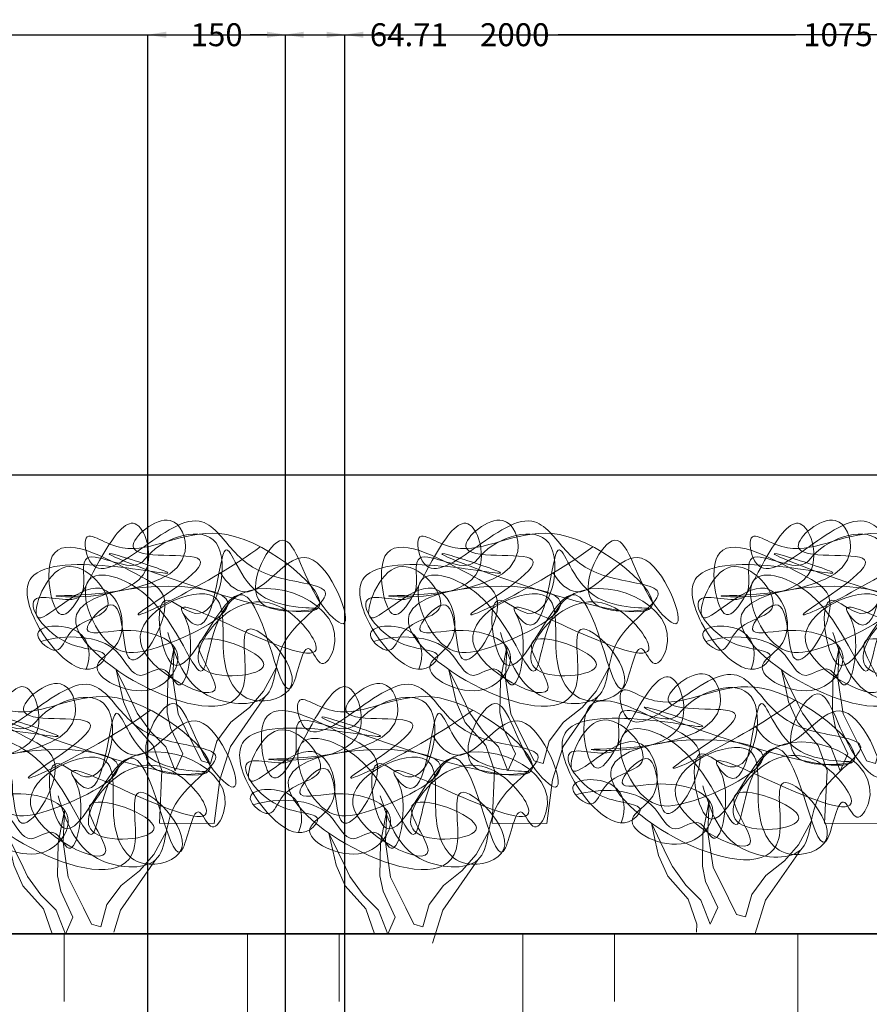
# Model space of a CAD drawing. Units: millimetres. Extents: x -692 to 9639, y -141 to 10345.
# Tile 16 of 19: x 3652 to 4578, y 9272 to 10345. Entities that reach past the tile are written whole.
import ezdxf

# ---------------------------------------------------------------- set-up
doc = ezdxf.new("R2010")
doc.units = ezdxf.units.MM
doc.header["$MEASUREMENT"] = 0
for name, color, linetype, lineweight in [('A-ANNO-DIMS', 2, 'Continuous', 18), ('A-ELEV', 7, 'Continuous', 35), ('A-ELEV-PATT', 8, 'Continuous', 13), ('L-PLNT', 3, 'Continuous', 18)]:
    doc.layers.add(name, color=color, linetype=linetype, lineweight=lineweight)
doc.styles.get("Standard").update_dxf_attribs({"font": 'arial.ttf'})
doc.dimstyles.get("Standard").update_dxf_attribs({"dimtxt": 25, "dimasz": 20, "dimexe": 0.18, "dimexo": 10, "dimgap": 10, "dimtad": 0, "dimtih": 1, "dimtoh": 1, "dimdec": 0, "dimzin": 0, "dimdsep": 46, "dimtxsty": 'Standard', "dimcen": 10, "dimadec": 0, "dimazin": 0, "dimtfac": 1, "dimtdec": 0, "dimtofl": 0, "dimtmove": 0, "dimatfit": 3, "dimfxl": 1, "dimtolj": 1, "dimtzin": 0, "dimarcsym": 0})

# ---------------------------------------------------------------- blocks, each defined once
blk = doc.blocks.new('SHRUB-A')
for p, q in [((56.2, 156.7), (63.1, 192.4)), ((63.1, 192.4), (61.6, 157.6)), ((4.3, 148.6), (0, 167.6)), ((0, 167.6), (10, 146.8)), ((160.6, 144.2), (174.3, 169.5)), ((55.6, 120.9), (56.2, 156.7)), ((61.6, 157.6), (67.3, 119.6)), ((7.9, 132.5), (4.3, 148.6)), ((10, 146.8), (18, 130.3)), ((145.1, 126.5), (160.6, 144.2)), ((17.8, 109.9), (7.9, 132.5)), ((18, 130.3), (22.9, 120.3)), ((162.4, 138.4), (124.4, 83.7)), ((22.9, 120.3), (37.4, 100.1)), ((59.1, 104.1), (55.6, 120.9)), ((67.3, 119.6), (83.9, 86)), ((124.8, 110.5), (145.1, 126.5)), ((40.2, 84.8), (17.8, 109.9)), ((109.4, 89.7), (124.8, 110.5)), ((37.4, 100.1), (54, 83.6)), ((72.4, 75.8), (59.1, 104.1)), ((83.9, 86), (92.7, 68.2)), ((102.6, 65.4), (109.4, 89.7)), ((49.7, 57.7), (40.2, 84.8)), ((54, 83.6), (64.1, 57.4)), ((64.1, 57.4), (72.4, 75.8)), ((124.4, 83.7), (113, 47.4)), ((92.7, 68.2), (102.6, 65.4)), ((47, 0.4), (49.7, 57.7)), ((113, 47.4), (106.7, 0)), ((106.7, 0), (47, 0.4))]:
    blk.add_line(p, q)
blk = doc.blocks.new('SHRUB-B')
for p, q in [((56.2, 99.2), (63.1, 135)), ((63.1, 135), (61.6, 100.2)), ((4.3, 91.2), (0, 110.2)), ((0, 110.2), (10, 89.4)), ((160.6, 86.8), (174.3, 112.1)), ((55.6, 63.5), (56.2, 99.2)), ((61.6, 100.2), (67.3, 62.2)), ((7.9, 75.1), (4.3, 91.2)), ((10, 89.4), (18, 72.9)), ((145.1, 69.1), (160.6, 86.8)), ((17.8, 52.5), (7.9, 75.1)), ((18, 72.9), (22.9, 62.9)), ((124.8, 53.1), (145.1, 69.1)), ((22.9, 62.9), (37.4, 42.7)), ((59.1, 46.7), (55.6, 63.5)), ((67.3, 62.2), (83.9, 28.6)), ((40.2, 27.4), (17.8, 52.5)), ((72.4, 18.4), (59.1, 46.7)), ((109.4, 32.3), (124.8, 53.1)), ((37.4, 42.7), (54, 26.2)), ((102.6, 8), (109.4, 32.3)), ((49.7, 0.3), (40.2, 27.4)), ((54, 26.2), (64.1, 0)), ((83.9, 28.6), (92.7, 10.8)), ((64.1, 0), (72.4, 18.4)), ((92.7, 10.8), (102.6, 8))]:
    blk.add_line(p, q)
blk = doc.blocks.new('*D7')
at = {"layer": 'A-ANNO-DIMS', "color": 0, "lineweight": -2, "transparency": 16777216}
for p, q in [((8481.5, 9848.8), (-649.1, 9848.8)), ((-648.9, 9828.8), (-648.9, 5124.9)), ((-648.9, 375.6), (-648.9, 5079.4)), ((2463.7, 355.6), (-649.1, 355.6))]:
    blk.add_line(p, q, dxfattribs=at)
at = {"layer": 'A-ANNO-DIMS', "color": 0, "lineweight": -3, "transparency": 16777216}
for points in [[(-652.2, 9828.8), (-645.6, 9828.8), (-648.9, 9848.8)], [(-652.2, 375.6), (-645.6, 375.6), (-648.9, 355.6)]]:
    blk.add_solid(points, dxfattribs=at)
at = {"layer": 'Defpoints', "color": 0, "lineweight": -3, "transparency": 16777216}
for p in [(-648.9, 9848.8), (8491.5, 9848.8), (2473.7, 355.6)]:
    blk.add_point(p, dxfattribs=at)
at = {"layer": 'A-ANNO-DIMS', "color": 0, "transparency": 16777216, "insert": (-648.9, 5102.2), "char_height": 25, "attachment_point": 5}
blk.add_mtext('\\A1;9493', dxfattribs=at)
blk = doc.blocks.new('*D14')
at = {"layer": 'A-ANNO-DIMS', "color": 0, "lineweight": -2, "transparency": 16777216}
for p, q in [((3191.5, 9358.8), (3191.5, 10329)), ((3211.5, 10328.8), (4144, 10328.8)), ((5171.5, 10328.8), (4239, 10328.8)), ((5191.5, 9358.8), (5191.5, 10329))]:
    blk.add_line(p, q, dxfattribs=at)
at = {"layer": 'A-ANNO-DIMS', "color": 0, "lineweight": -3, "transparency": 16777216}
for points in [[(3211.5, 10332.1), (3211.5, 10325.4), (3191.5, 10328.8)], [(5171.5, 10332.1), (5171.5, 10325.4), (5191.5, 10328.8)]]:
    blk.add_solid(points, dxfattribs=at)
at = {"layer": 'Defpoints', "color": 0, "lineweight": -3, "transparency": 16777216}
for p in [(5191.5, 10328.8), (3191.5, 9348.8), (5191.5, 9348.8)]:
    blk.add_point(p, dxfattribs=at)
at = {"layer": 'A-ANNO-DIMS', "color": 0, "transparency": 16777216, "insert": (4191.5, 10328.8), "char_height": 25, "attachment_point": 5}
blk.add_mtext('\\A1;2000', dxfattribs=at)
blk = doc.blocks.new('*D52')
at = {"layer": 'A-ANNO-DIMS', "color": 0, "lineweight": -2, "transparency": 16777216}
for p, q in [((3791.5, 6858.8), (3791.5, 10329)), ((3811.5, 10328.8), (3830.1, 10328.8)), ((3921.5, 10328.8), (3902.9, 10328.8)), ((3941.5, 6708.8), (3941.5, 10329))]:
    blk.add_line(p, q, dxfattribs=at)
at = {"layer": 'A-ANNO-DIMS', "color": 0, "lineweight": -3, "transparency": 16777216}
for points in [[(3811.5, 10332.1), (3811.5, 10325.4), (3791.5, 10328.8)], [(3921.5, 10332.1), (3921.5, 10325.4), (3941.5, 10328.8)]]:
    blk.add_solid(points, dxfattribs=at)
at = {"layer": 'Defpoints', "color": 0, "lineweight": -3, "transparency": 16777216}
for p in [(3941.5, 10328.8), (3791.5, 6848.8), (3941.5, 6698.8)]:
    blk.add_point(p, dxfattribs=at)
at = {"layer": 'A-ANNO-DIMS', "color": 0, "transparency": 16777216, "insert": (3866.5, 10328.8), "char_height": 25, "attachment_point": 5}
blk.add_mtext('\\A1;150', dxfattribs=at)
blk = doc.blocks.new('*D53')
at = {"layer": 'A-ANNO-DIMS', "color": 0, "lineweight": -2, "transparency": 16777216}
for p, q in [((3941.5, 6708.8), (3941.5, 10329)), ((3961.5, 10328.8), (3986.3, 10328.8)), ((4006.3, 6433.8), (4006.3, 10329)), ((4006.3, 10328.8), (4026.3, 10328.8))]:
    blk.add_line(p, q, dxfattribs=at)
at = {"layer": 'A-ANNO-DIMS', "color": 0, "lineweight": -3, "transparency": 16777216}
for points in [[(3961.5, 10332.1), (3961.5, 10325.4), (3941.5, 10328.8)], [(3986.3, 10332.1), (3986.3, 10325.4), (4006.3, 10328.8)]]:
    blk.add_solid(points, dxfattribs=at)
at = {"layer": 'Defpoints', "color": 0, "lineweight": -3, "transparency": 16777216}
for p in [(4006.3, 10328.8), (3941.5, 6698.8), (4006.3, 6423.8)]:
    blk.add_point(p, dxfattribs=at)
at = {"layer": 'A-ANNO-DIMS', "color": 0, "transparency": 16777216, "insert": (4076.1, 10328.8), "char_height": 25, "attachment_point": 5}
blk.add_mtext('\\A1;64.71', dxfattribs=at)
blk = doc.blocks.new('*D54')
at = {"layer": 'A-ANNO-DIMS', "color": 0, "lineweight": -2, "transparency": 16777216}
for p, q in [((4006.3, 6433.8), (4006.3, 10329)), ((4026.3, 10328.8), (4497.5, 10328.8)), ((5061.3, 10328.8), (4590, 10328.8)), ((5081.3, 6433.8), (5081.3, 10329))]:
    blk.add_line(p, q, dxfattribs=at)
at = {"layer": 'A-ANNO-DIMS', "color": 0, "lineweight": -3, "transparency": 16777216}
for points in [[(4026.3, 10332.1), (4026.3, 10325.4), (4006.3, 10328.8)], [(5061.3, 10332.1), (5061.3, 10325.4), (5081.3, 10328.8)]]:
    blk.add_solid(points, dxfattribs=at)
at = {"layer": 'Defpoints', "color": 0, "lineweight": -3, "transparency": 16777216}
for p in [(5081.3, 10328.8), (4006.3, 6423.8), (5081.3, 6423.8)]:
    blk.add_point(p, dxfattribs=at)
at = {"layer": 'A-ANNO-DIMS', "color": 0, "transparency": 16777216, "insert": (4543.8, 10328.8), "char_height": 25, "attachment_point": 5}
blk.add_mtext('\\A1;1075', dxfattribs=at)

msp = doc.modelspace()

# ---------------------------------------------------------------- hatches: boundary and pattern name
at = {"layer": 'A-ELEV-PATT'}
h = msp.add_hatch(dxfattribs=at)
h.set_pattern_fill('GOST_WOOD', color=256, scale=50)
h.set_pattern_definition([(90, (0, 0), (300, -2e-14), [500, -100]), (90, (100, -100), (300, -2e-14), [300, -75, 150, -75]), (90, (200, -250), (300, -2e-14), [500, -100])])
edge = h.paths.add_edge_path()
edge.add_line((5191.547, 8748.772), (3791.547, 8748.772))
edge.add_line((3791.547, 8748.772), (3791.547, 8848.772))
edge.add_line((3791.547, 8848.772), (5191.547, 8848.772))
edge.add_line((5191.547, 8848.772), (5191.547, 9348.772))
edge.add_line((5191.547, 9348.772), (4755.992, 9348.772))
edge.add_line((4755.992, 9348.772), (4755.854, 9348.465))
edge.add_line((4755.854, 9348.465), (4755.734, 9348.772))
edge.add_line((4755.734, 9348.772), (4053.129, 9348.772))
edge.add_line((4053.129, 9348.772), (4052.99, 9348.465))
edge.add_line((4052.99, 9348.465), (4052.871, 9348.772))
edge.add_line((4052.871, 9348.772), (3701.731, 9348.772))
edge.add_line((3701.731, 9348.772), (3701.593, 9348.465))
edge.add_line((3701.593, 9348.465), (3701.474, 9348.772))
edge.add_line((3701.474, 9348.772), (3368.199, 9348.772))
edge.add_line((3368.199, 9348.772), (3368.061, 9348.465))
edge.add_line((3368.061, 9348.465), (3367.942, 9348.772))
edge.add_line((3367.942, 9348.772), (3191.547, 9348.772))
edge.add_line((3191.547, 9348.772), (3191.547, 3210.058))
edge.add_spline(control_points=[(3191.547, 3210.058), (3198.467, 3207.5), (3283.859, 3166.656), (3324.053, 2995.08), (3234.02, 2920.058), (3220.783, 2911.684)], knot_values=[13649.89756952, 13649.89756952, 13649.89756952, 13649.89756952, 13672.14990348, 13935.42377748, 13974.4426778, 13974.4426778, 13974.4426778, 13974.4426778], degree=3, periodic=0)
edge.add_spline(control_points=[(3220.783, 2911.684), (3225.148, 2890.107), (3226.864, 2868.931), (3226.144, 2848.27)], knot_values=[8828.69997321, 8828.69997321, 8828.69997321, 8828.69997321, 8890.6429847, 8890.6429847, 8890.6429847, 8890.6429847], degree=3, periodic=0)
edge.add_line((3226.144, 2848.27), (5191.547, 2848.27))
edge.add_line((5191.547, 2848.27), (5191.547, 3048.27))
edge.add_line((5191.547, 3048.27), (5041.547, 3048.27))
edge.add_line((5041.547, 3048.27), (5041.547, 3148.27))
edge.add_line((5041.547, 3148.27), (5091.547, 3148.27))
edge.add_line((5091.547, 3148.27), (5091.547, 3598.27))
edge.add_line((5091.547, 3598.27), (5191.547, 3598.27))
edge.add_line((5191.547, 3598.27), (5191.547, 4848.772))
edge.add_line((5191.547, 4848.772), (3791.547, 4848.772))
edge.add_line((3791.547, 4848.772), (3791.547, 6848.772))
edge.add_line((3791.547, 6848.772), (5091.547, 6848.772))
edge.add_line((5091.547, 6848.772), (5091.547, 7298.772))
edge.add_line((5091.547, 7298.772), (5191.547, 7298.772))
edge.add_line((5191.547, 7298.772), (5191.547, 8748.772))
h.paths.add_polyline_path([(5016.547, 8198.772), (5016.547, 7123.772), (3941.547, 7123.772), (3941.547, 8198.772)], flags=16)
h.paths.add_polyline_path([(4941.547, 8123.772), (4941.547, 7198.772), (4016.547, 7198.772), (4016.547, 8123.772)], flags=0)
h.paths.add_polyline_path([(4616.547, 8073.772), (4616.547, 7248.772), (4341.547, 7248.772), (4341.547, 8073.772)], flags=0)
h.paths.add_polyline_path([(4641.547, 8073.772), (4891.547, 8073.772), (4891.547, 7248.772), (4641.547, 7248.772)], flags=0)
h.paths.add_polyline_path([(4666.547, 8048.772), (4866.547, 8048.772), (4866.547, 7273.772), (4666.547, 7273.772)], flags=0)
h.paths.add_polyline_path([(4316.547, 8073.772), (4316.547, 7248.772), (4066.547, 7248.772), (4066.547, 8073.772)], flags=0)
h.paths.add_polyline_path([(4291.547, 8048.772), (4291.547, 7273.772), (4091.547, 7273.772), (4091.547, 8048.772)], flags=0)
h.paths.add_polyline_path([(5016.547, 4497.772), (5016.547, 3422.772), (3941.547, 3422.772), (3941.547, 4497.772)], flags=16)
h.paths.add_polyline_path([(4941.547, 4422.772), (4941.547, 3497.772), (4016.547, 3497.772), (4016.547, 4422.772)], flags=0)
h.paths.add_polyline_path([(4616.547, 4372.772), (4616.547, 3547.772), (4341.547, 3547.772), (4341.547, 4372.772)], flags=0)
h.paths.add_polyline_path([(4641.547, 4372.772), (4891.547, 4372.772), (4891.547, 3547.772), (4641.547, 3547.772)], flags=0)
h.paths.add_polyline_path([(4316.547, 4372.772), (4316.547, 3547.772), (4066.547, 3547.772), (4066.547, 4372.772)], flags=0)
h.paths.add_polyline_path([(4666.547, 4347.772), (4866.547, 4347.772), (4866.547, 3572.772), (4666.547, 3572.772)], flags=0)
h.paths.add_polyline_path([(4291.547, 4347.772), (4291.547, 3572.772), (4091.547, 3572.772), (4091.547, 4347.772)], flags=0)

# ---------------------------------------------------------------- linework, layer by layer
at = {"layer": 'A-ELEV'}
msp.add_line((3191.547, 9348.772), (5191.547, 9348.772), dxfattribs=at)
at = {"layer": 'L-PLNT'}
for p, q in [((4396.605, 9458.408), (4403.593, 9494.115)), ((4403.593, 9494.115), (4402.028, 9459.362)), ((4344.728, 9450.331), (4340.453, 9469.321)), ((4340.453, 9469.321), (4350.494, 9448.579)), ((4501.01, 9445.975), (4514.74, 9471.226)), ((4396.049, 9422.669), (4396.605, 9458.408)), ((4402.028, 9459.362), (4407.8, 9421.335)), ((4348.34, 9434.283), (4344.728, 9450.331)), ((4350.494, 9448.579), (4358.483, 9432.077)), ((4485.516, 9428.273), (4501.01, 9445.975)), ((4358.252, 9411.658), (4348.34, 9434.283)), ((4502.899, 9440.134), (4464.833, 9385.403)), ((3799.897, 9429.44), (3761.831, 9374.709)), ((4151.294, 9429.44), (4113.229, 9374.709)), ((4358.483, 9432.077), (4363.315, 9422.096)), ((4465.219, 9412.262), (4485.516, 9428.273)), ((4363.315, 9422.096), (4377.888, 9401.855)), ((4399.52, 9405.858), (4396.049, 9422.669)), ((4407.8, 9421.335), (4424.358, 9387.712)), ((4449.855, 9391.498), (4465.219, 9412.262)), ((4380.638, 9386.579), (4358.252, 9411.658)), ((4377.888, 9401.855), (4394.446, 9385.31)), ((4412.874, 9377.572), (4399.52, 9405.858)), ((4443.052, 9367.164), (4449.855, 9391.498)), ((4390.135, 9359.466), (4380.638, 9386.579)), ((4394.446, 9385.31), (4404.595, 9359.159)), ((4424.358, 9387.712), (4433.107, 9369.945)), ((4464.833, 9385.403), (4453.484, 9349.201)), ((3761.831, 9374.709), (3754.255, 9350.541)), ((4113.229, 9374.709), (4101.88, 9338.507)), ((4404.595, 9359.159), (4412.874, 9377.572)), ((4433.107, 9369.945), (4443.052, 9367.164)), ((4389.721, 9350.541), (4390.135, 9359.466))]:
    msp.add_line(p, q, dxfattribs=at)
for points, knots in [([(3870.787, 9742.239), (3877.292, 9730.903), (3910.528, 9700.951), (3966.958, 9812.559), (4026.138, 9660.867), (3961.502, 9722.363), (3945.777, 9821.568), (3878.818, 9687.955), (4016.284, 9708.276), (3899.439, 9697.909), (3870.103, 9822.951), (3864.501, 9656.273), (3811.999, 9718.176), (3905.68, 9672.588), (4002.746, 9634.5), (3933.585, 9723.816), (3867.431, 9704.087), (3825.22, 9620.458), (3976.108, 9634.855), (3810.499, 9696.668), (3906.873, 9576.858), (3713.031, 9670.533), (3887.727, 9749.582), (3865.518, 9651.408), (3894.256, 9592.145), (3980.508, 9617.027), (3878.674, 9721.539), (3933.88, 9522.359), (3548.286, 9733.486), (3963.38, 9736.751), (3813.397, 9659.817), (3742.545, 9649.423), (3699.733, 9757.262), (3814.514, 9723.536), (3856.602, 9579.097), (3861.587, 9768.661), (4023.281, 9702.629), (3980.554, 9633.263), (3962.517, 9680.84), (3941.722, 9544.945), (3904.968, 9826.86), (3817.837, 9563.572), (3792.835, 9739.876), (3862.604, 9668.929), (3894.271, 9809.339), (3803.73, 9778.979), (3774.605, 9737.949), (3707.662, 9784.348), (3733.853, 9697.774), (3641.411, 9733.91), (3691.228, 9654.8), (3752.747, 9658.957), (3722.581, 9620.328), (3667.277, 9675.174), (3642.995, 9782.065), (3887.369, 9719.852), (3639.078, 9801.027), (4099.827, 9622.054), (3874.162, 9821.297), (3794.319, 9760.575), (3748.016, 9773.261), (3719.932, 9789.116), (3732.294, 9699.252), (3833.622, 9839.527), (3885.762, 9759.776), (3924.577, 9734.293), (4016.253, 9726.404), (3923.236, 9674.075), (3937.396, 9593.308), (3837.579, 9601.408), (3821.952, 9650.09), (3813.209, 9677.329)], [2413.81083439, 2413.81083439, 2413.81083439, 2413.81083439, 2446.13175162, 2525.76080664, 2606.35842411, 2641.00152553, 2720.74212251, 2790.99014926, 2851.81652626, 2913.32865241, 2976.26621652, 3063.90114016, 3082.75198237, 3142.42040078, 3234.21047015, 3290.89514405, 3366.44484787, 3415.98940505, 3483.69911772, 3557.93307926, 3609.73318023, 3705.73947781, 3799.4035149, 3865.9559372, 3923.0506034, 3967.47996902, 4044.49288828, 4106.44083814, 4304.51898163, 4470.20683119, 4567.66187689, 4605.3795614, 4686.71522755, 4750.59418277, 4853.67923318, 4940.38216709, 5061.92671957, 5081.75583403, 5102.38342504, 5145.20608443, 5257.20859169, 5364.77120979, 5434.601162, 5468.93345211, 5548.91442162, 5624.29444335, 5636.24531967, 5696.20028889, 5735.53268567, 5783.76480276, 5846.42206129, 5886.03768999, 5892.5373904, 5975.51315878, 6025.10951571, 6171.93373357, 6229.50952465, 6457.88730992, 6585.61219414, 6694.59236697, 6720.94216912, 6740.48817363, 6762.80712224, 6890.45590486, 6938.76737224, 6996.52597549, 7050.2147859, 7119.04318667, 7183.57042671, 7247.02609863, 7327.63038966, 7327.63038966, 7327.63038966, 7327.63038966]), ([(3724.096, 9637.137), (3730.159, 9651.341), (3726.664, 9689.445), (3652.093, 9684.583), (3695.541, 9647.305), (3706.222, 9691.38), (3775.283, 9694.456), (3695.331, 9786.768), (3646.836, 9649.897), (3745.311, 9765.156), (3777.086, 9667.558), (3713.033, 9636.75), (3795.836, 9595.485), (3843.182, 9663.04), (3778.736, 9686.864), (3708.195, 9669.411), (3769.699, 9738.522), (3756.754, 9597.689), (3831.066, 9714.368), (3765.302, 9747.322), (3669.526, 9801.44), (3693.692, 9656.882), (3733.265, 9753.527), (3780.402, 9818.105), (3813.993, 9708.231), (3585.245, 9723.215), (3859.393, 9710.208), (3819.392, 9819.441), (3735.993, 9748.74), (3911.027, 9777.439), (3699.503, 9652.419), (3863.756, 9733.103), (3913.888, 9770.678)], [369.05069933, 369.05069933, 369.05069933, 369.05069933, 408.0755152, 451.81999766, 477.70991819, 501.76804774, 551.72688153, 614.71506468, 677.59190345, 752.65992621, 814.92518896, 848.06947292, 911.78367098, 957.89252981, 1028.01014559, 1063.15062915, 1099.93333455, 1162.00574744, 1235.23981988, 1278.45742209, 1371.86548038, 1434.47491944, 1513.90135623, 1562.79289697, 1613.81915843, 1716.27616866, 1864.9556669, 1902.31221643, 1951.61463942, 2025.20033993, 2111.30740148, 2244.75178922, 2244.75178922, 2244.75178922, 2244.75178922]), ([(4233.453, 9742.239), (4239.959, 9730.903), (4273.195, 9700.951), (4329.624, 9812.559), (4388.805, 9660.867), (4324.169, 9722.363), (4308.443, 9821.568), (4241.484, 9687.955), (4378.95, 9708.276), (4262.105, 9697.909), (4232.77, 9822.951), (4227.167, 9656.273), (4174.665, 9718.176), (4268.346, 9672.588), (4365.412, 9634.5), (4296.251, 9723.816), (4230.098, 9704.087), (4187.887, 9620.458), (4338.774, 9634.855), (4173.165, 9696.668), (4269.539, 9576.858), (4075.697, 9670.533), (4250.394, 9749.582), (4228.185, 9651.408), (4256.922, 9592.145), (4343.175, 9617.027), (4241.341, 9721.539), (4296.546, 9522.359), (3910.953, 9733.486), (4326.046, 9736.751), (4176.063, 9659.817), (4105.212, 9649.423), (4062.399, 9757.262), (4177.18, 9723.536), (4219.268, 9579.097), (4224.254, 9768.661), (4385.947, 9702.629), (4343.22, 9633.263), (4325.183, 9680.84), (4304.388, 9544.945), (4267.634, 9826.86), (4180.503, 9563.572), (4155.501, 9739.876), (4225.27, 9668.929), (4256.937, 9809.339), (4166.397, 9778.979), (4137.271, 9737.949), (4070.329, 9784.348), (4096.519, 9697.774), (4004.078, 9733.91), (4053.894, 9654.8), (4115.414, 9658.957), (4085.247, 9620.328), (4029.943, 9675.174), (4005.662, 9782.065), (4250.036, 9719.852), (4001.744, 9801.027), (4462.493, 9622.054), (4236.829, 9821.297), (4156.985, 9760.575), (4110.682, 9773.261), (4082.599, 9789.116), (4094.96, 9699.252), (4196.289, 9839.527), (4248.429, 9759.776), (4287.243, 9734.293), (4378.919, 9726.404), (4285.902, 9674.075), (4300.063, 9593.308), (4200.245, 9601.408), (4184.619, 9650.09), (4175.875, 9677.329)], [2413.81083439, 2413.81083439, 2413.81083439, 2413.81083439, 2446.13175162, 2525.76080664, 2606.35842411, 2641.00152553, 2720.74212251, 2790.99014926, 2851.81652626, 2913.32865241, 2976.26621652, 3063.90114016, 3082.75198237, 3142.42040078, 3234.21047015, 3290.89514405, 3366.44484787, 3415.98940505, 3483.69911772, 3557.93307926, 3609.73318023, 3705.73947781, 3799.4035149, 3865.9559372, 3923.0506034, 3967.47996902, 4044.49288828, 4106.44083814, 4304.51898163, 4470.20683119, 4567.66187689, 4605.3795614, 4686.71522755, 4750.59418277, 4853.67923318, 4940.38216709, 5061.92671957, 5081.75583403, 5102.38342504, 5145.20608443, 5257.20859169, 5364.77120979, 5434.601162, 5468.93345211, 5548.91442162, 5624.29444335, 5636.24531967, 5696.20028889, 5735.53268567, 5783.76480276, 5846.42206129, 5886.03768999, 5892.5373904, 5975.51315878, 6025.10951571, 6171.93373357, 6229.50952465, 6457.88730992, 6585.61219414, 6694.59236697, 6720.94216912, 6740.48817363, 6762.80712224, 6890.45590486, 6938.76737224, 6996.52597549, 7050.2147859, 7119.04318667, 7183.57042671, 7247.02609863, 7327.63038966, 7327.63038966, 7327.63038966, 7327.63038966]), ([(4086.762, 9637.137), (4092.825, 9651.341), (4089.331, 9689.445), (4014.759, 9684.583), (4058.207, 9647.305), (4068.889, 9691.38), (4137.95, 9694.456), (4057.998, 9786.768), (4009.502, 9649.897), (4107.978, 9765.156), (4139.753, 9667.558), (4075.699, 9636.75), (4158.502, 9595.485), (4205.849, 9663.04), (4141.402, 9686.864), (4070.861, 9669.411), (4132.366, 9738.522), (4119.421, 9597.689), (4193.732, 9714.368), (4127.969, 9747.322), (4032.193, 9801.44), (4056.358, 9656.882), (4095.932, 9753.527), (4143.068, 9818.105), (4176.659, 9708.231), (3947.911, 9723.215), (4222.059, 9710.208), (4182.058, 9819.441), (4098.659, 9748.74), (4273.694, 9777.439), (4062.17, 9652.419), (4226.423, 9733.103), (4276.554, 9770.678)], [369.05069933, 369.05069933, 369.05069933, 369.05069933, 408.0755152, 451.81999766, 477.70991819, 501.76804774, 551.72688153, 614.71506468, 677.59190345, 752.65992621, 814.92518896, 848.06947292, 911.78367098, 957.89252981, 1028.01014559, 1063.15062915, 1099.93333455, 1162.00574744, 1235.23981988, 1278.45742209, 1371.86548038, 1434.47491944, 1513.90135623, 1562.79289697, 1613.81915843, 1716.27616866, 1864.9556669, 1902.31221643, 1951.61463942, 2025.20033993, 2111.30740148, 2244.75178922, 2244.75178922, 2244.75178922, 2244.75178922]), ([(4595.897, 9742.239), (4602.402, 9730.903), (4635.638, 9700.951), (4692.068, 9812.559), (4751.248, 9660.867), (4686.612, 9722.363), (4670.887, 9821.568), (4603.928, 9687.955), (4741.394, 9708.276), (4624.549, 9697.909), (4595.213, 9822.951), (4589.611, 9656.273), (4537.109, 9718.176), (4630.79, 9672.588), (4727.856, 9634.5), (4658.695, 9723.816), (4592.541, 9704.087), (4550.33, 9620.458), (4701.218, 9634.855), (4535.609, 9696.668), (4631.983, 9576.858), (4438.141, 9670.533), (4612.837, 9749.582), (4590.628, 9651.408), (4619.366, 9592.145), (4705.618, 9617.027), (4603.784, 9721.539), (4658.99, 9522.359), (4273.396, 9733.486), (4688.49, 9736.751), (4538.507, 9659.817), (4467.655, 9649.423), (4424.843, 9757.262), (4539.624, 9723.536), (4581.712, 9579.097), (4586.697, 9768.661), (4748.391, 9702.629), (4705.664, 9633.263), (4687.627, 9680.84), (4666.832, 9544.945), (4630.078, 9826.86), (4542.947, 9563.572), (4517.945, 9739.876), (4587.714, 9668.929), (4619.381, 9809.339), (4528.84, 9778.979), (4499.715, 9737.949), (4432.772, 9784.348), (4458.963, 9697.774), (4366.521, 9733.91), (4416.338, 9654.8), (4477.857, 9658.957), (4447.691, 9620.328), (4392.387, 9675.174), (4368.105, 9782.065), (4612.479, 9719.852), (4364.188, 9801.027), (4824.937, 9622.054), (4599.272, 9821.297), (4519.429, 9760.575), (4473.126, 9773.261), (4445.042, 9789.116), (4457.404, 9699.252), (4558.733, 9839.527), (4610.872, 9759.776), (4649.687, 9734.293), (4741.363, 9726.404), (4648.346, 9674.075), (4662.506, 9593.308), (4562.689, 9601.408), (4547.062, 9650.09), (4538.319, 9677.329)], [2413.81083439, 2413.81083439, 2413.81083439, 2413.81083439, 2446.13175162, 2525.76080664, 2606.35842411, 2641.00152553, 2720.74212251, 2790.99014926, 2851.81652626, 2913.32865241, 2976.26621652, 3063.90114016, 3082.75198237, 3142.42040078, 3234.21047015, 3290.89514405, 3366.44484787, 3415.98940505, 3483.69911772, 3557.93307926, 3609.73318023, 3705.73947781, 3799.4035149, 3865.9559372, 3923.0506034, 3967.47996902, 4044.49288828, 4106.44083814, 4304.51898163, 4470.20683119, 4567.66187689, 4605.3795614, 4686.71522755, 4750.59418277, 4853.67923318, 4940.38216709, 5061.92671957, 5081.75583403, 5102.38342504, 5145.20608443, 5257.20859169, 5364.77120979, 5434.601162, 5468.93345211, 5548.91442162, 5624.29444335, 5636.24531967, 5696.20028889, 5735.53268567, 5783.76480276, 5846.42206129, 5886.03768999, 5892.5373904, 5975.51315878, 6025.10951571, 6171.93373357, 6229.50952465, 6457.88730992, 6585.61219414, 6694.59236697, 6720.94216912, 6740.48817363, 6762.80712224, 6890.45590486, 6938.76737224, 6996.52597549, 7050.2147859, 7119.04318667, 7183.57042671, 7247.02609863, 7327.63038966, 7327.63038966, 7327.63038966, 7327.63038966]), ([(4449.206, 9637.137), (4455.269, 9651.341), (4451.774, 9689.445), (4377.203, 9684.583), (4420.651, 9647.305), (4431.332, 9691.38), (4500.393, 9694.456), (4420.441, 9786.768), (4371.946, 9649.897), (4470.421, 9765.156), (4502.196, 9667.558), (4438.143, 9636.75), (4520.946, 9595.485), (4568.292, 9663.04), (4503.846, 9686.864), (4433.305, 9669.411), (4494.809, 9738.522), (4481.865, 9597.689), (4556.176, 9714.368), (4490.412, 9747.322), (4394.637, 9801.44), (4418.802, 9656.882), (4458.375, 9753.527), (4505.512, 9818.105), (4539.103, 9708.231), (4310.355, 9723.215), (4584.503, 9710.208), (4544.502, 9819.441), (4461.103, 9748.74), (4636.137, 9777.439), (4424.613, 9652.419), (4588.866, 9733.103), (4638.998, 9770.678)], [369.05069933, 369.05069933, 369.05069933, 369.05069933, 408.0755152, 451.81999766, 477.70991819, 501.76804774, 551.72688153, 614.71506468, 677.59190345, 752.65992621, 814.92518896, 848.06947292, 911.78367098, 957.89252981, 1028.01014559, 1063.15062915, 1099.93333455, 1162.00574744, 1235.23981988, 1278.45742209, 1371.86548038, 1434.47491944, 1513.90135623, 1562.79289697, 1613.81915843, 1716.27616866, 1864.9556669, 1902.31221643, 1951.61463942, 2025.20033993, 2111.30740148, 2244.75178922, 2244.75178922, 2244.75178922, 2244.75178922]), ([(3828.816, 9700.071), (3832.306, 9693.404), (3843.803, 9671.444), (3830.732, 9597.516), (3809.551, 9646.949), (3776.741, 9618.501), (3759.154, 9674.749), (3701.401, 9675.405), (3674.69, 9667.541)], [0, 0, 0, 0, 24.87287104, 81.92705424, 103.09014331, 128.64171207, 165.87657864, 231.33124244, 231.33124244, 231.33124244, 231.33124244]), ([(4191.483, 9700.071), (4194.973, 9693.404), (4206.47, 9671.444), (4193.399, 9597.516), (4172.217, 9646.949), (4139.407, 9618.501), (4121.821, 9674.749), (4064.068, 9675.405), (4037.356, 9667.541)], [0, 0, 0, 0, 24.87287104, 81.92705424, 103.09014331, 128.64171207, 165.87657864, 231.33124244, 231.33124244, 231.33124244, 231.33124244]), ([(4553.926, 9700.071), (4557.417, 9693.404), (4568.913, 9671.444), (4555.842, 9597.516), (4534.661, 9646.949), (4501.851, 9618.501), (4484.264, 9674.749), (4426.511, 9675.405), (4399.8, 9667.541)], [0, 0, 0, 0, 24.87287104, 81.92705424, 103.09014331, 128.64171207, 165.87657864, 231.33124244, 231.33124244, 231.33124244, 231.33124244]), ([(4454.121, 9574.89), (4460.627, 9563.555), (4493.863, 9533.603), (4550.293, 9645.211), (4609.473, 9493.518), (4544.837, 9555.014), (4529.111, 9654.219), (4462.152, 9520.607), (4599.618, 9540.927), (4482.774, 9530.56), (4453.438, 9655.602), (4447.835, 9488.925), (4395.334, 9550.827), (4489.014, 9505.239), (4586.08, 9467.152), (4516.919, 9556.467), (4450.766, 9536.738), (4408.555, 9453.11), (4559.442, 9467.506), (4393.833, 9529.319), (4490.208, 9409.509), (4296.366, 9503.184), (4471.062, 9582.233), (4448.853, 9484.06), (4477.59, 9424.796), (4563.843, 9449.679), (4462.009, 9554.19), (4517.215, 9355.01), (4131.621, 9566.137), (4546.715, 9569.402), (4396.732, 9492.468), (4325.88, 9482.075), (4283.067, 9589.914), (4397.848, 9556.187), (4439.936, 9411.748), (4444.922, 9601.313), (4606.615, 9535.28), (4563.888, 9465.914), (4545.851, 9513.492), (4525.056, 9377.596), (4488.303, 9659.511), (4401.171, 9396.224), (4376.169, 9572.528), (4445.938, 9501.581), (4477.605, 9641.99), (4387.065, 9611.631), (4357.939, 9570.6), (4290.997, 9617), (4317.188, 9530.425), (4224.746, 9566.561), (4274.562, 9487.452), (4336.082, 9491.609), (4305.915, 9452.98), (4250.611, 9507.825), (4226.33, 9614.716), (4470.704, 9552.503), (4222.412, 9633.678), (4683.161, 9454.705), (4457.497, 9653.948), (4377.653, 9593.226), (4331.351, 9605.912), (4303.267, 9621.768), (4315.629, 9531.903), (4416.957, 9672.178), (4469.097, 9592.428), (4507.911, 9566.944), (4599.587, 9559.055), (4506.57, 9506.727), (4520.731, 9425.959), (4420.913, 9434.059), (4405.287, 9482.742), (4396.543, 9509.98)], [2413.81083439, 2413.81083439, 2413.81083439, 2413.81083439, 2446.13175162, 2525.76080664, 2606.35842411, 2641.00152553, 2720.74212251, 2790.99014926, 2851.81652626, 2913.32865241, 2976.26621652, 3063.90114016, 3082.75198237, 3142.42040078, 3234.21047015, 3290.89514405, 3366.44484787, 3415.98940505, 3483.69911772, 3557.93307926, 3609.73318023, 3705.73947781, 3799.4035149, 3865.9559372, 3923.0506034, 3967.47996902, 4044.49288828, 4106.44083814, 4304.51898163, 4470.20683119, 4567.66187689, 4605.3795614, 4686.71522755, 4750.59418277, 4853.67923318, 4940.38216709, 5061.92671957, 5081.75583403, 5102.38342504, 5145.20608443, 5257.20859169, 5364.77120979, 5434.601162, 5468.93345211, 5548.91442162, 5624.29444335, 5636.24531967, 5696.20028889, 5735.53268567, 5783.76480276, 5846.42206129, 5886.03768999, 5892.5373904, 5975.51315878, 6025.10951571, 6171.93373357, 6229.50952465, 6457.88730992, 6585.61219414, 6694.59236697, 6720.94216912, 6740.48817363, 6762.80712224, 6890.45590486, 6938.76737224, 6996.52597549, 7050.2147859, 7119.04318667, 7183.57042671, 7247.02609863, 7327.63038966, 7327.63038966, 7327.63038966, 7327.63038966]), ([(3751.119, 9564.196), (3757.625, 9552.861), (3790.861, 9522.909), (3847.291, 9634.516), (3906.471, 9482.824), (3841.835, 9544.32), (3826.109, 9643.525), (3759.15, 9509.913), (3896.616, 9530.233), (3779.772, 9519.866), (3750.436, 9644.908), (3744.834, 9478.231), (3692.332, 9540.133), (3786.013, 9494.545), (3883.078, 9456.457), (3813.917, 9545.773), (3747.764, 9526.044), (3705.553, 9442.416), (3856.44, 9456.812), (3690.831, 9518.625), (3787.206, 9398.815), (3593.364, 9492.49), (3768.06, 9571.539), (3745.851, 9473.365), (3774.589, 9414.102), (3860.841, 9438.984), (3759.007, 9543.496), (3814.213, 9344.316), (3428.619, 9555.443), (3843.713, 9558.708), (3693.73, 9481.774), (3622.878, 9471.381), (3580.065, 9579.22), (3694.847, 9545.493), (3736.934, 9401.054), (3741.92, 9590.618), (3903.613, 9524.586), (3860.886, 9455.22), (3842.849, 9502.798), (3822.054, 9366.902), (3785.301, 9648.817), (3698.169, 9385.529), (3673.168, 9561.834), (3742.936, 9490.886), (3774.603, 9631.296), (3684.063, 9600.937), (3654.937, 9559.906), (3587.995, 9606.306), (3614.186, 9519.731), (3521.744, 9555.867), (3571.56, 9476.758), (3633.08, 9480.914), (3602.913, 9442.286), (3547.609, 9497.131), (3523.328, 9604.022), (3767.702, 9541.809), (3519.41, 9622.984), (3980.16, 9444.011), (3754.495, 9643.254), (3674.651, 9582.532), (3628.349, 9595.218), (3600.265, 9611.073), (3612.627, 9521.209), (3713.955, 9661.484), (3766.095, 9581.734), (3804.909, 9556.25), (3896.585, 9548.361), (3803.568, 9496.032), (3817.729, 9415.265), (3717.911, 9423.365), (3702.285, 9472.047), (3693.541, 9499.286)], [2413.81083439, 2413.81083439, 2413.81083439, 2413.81083439, 2446.13175162, 2525.76080664, 2606.35842411, 2641.00152553, 2720.74212251, 2790.99014926, 2851.81652626, 2913.32865241, 2976.26621652, 3063.90114016, 3082.75198237, 3142.42040078, 3234.21047015, 3290.89514405, 3366.44484787, 3415.98940505, 3483.69911772, 3557.93307926, 3609.73318023, 3705.73947781, 3799.4035149, 3865.9559372, 3923.0506034, 3967.47996902, 4044.49288828, 4106.44083814, 4304.51898163, 4470.20683119, 4567.66187689, 4605.3795614, 4686.71522755, 4750.59418277, 4853.67923318, 4940.38216709, 5061.92671957, 5081.75583403, 5102.38342504, 5145.20608443, 5257.20859169, 5364.77120979, 5434.601162, 5468.93345211, 5548.91442162, 5624.29444335, 5636.24531967, 5696.20028889, 5735.53268567, 5783.76480276, 5846.42206129, 5886.03768999, 5892.5373904, 5975.51315878, 6025.10951571, 6171.93373357, 6229.50952465, 6457.88730992, 6585.61219414, 6694.59236697, 6720.94216912, 6740.48817363, 6762.80712224, 6890.45590486, 6938.76737224, 6996.52597549, 7050.2147859, 7119.04318667, 7183.57042671, 7247.02609863, 7327.63038966, 7327.63038966, 7327.63038966, 7327.63038966]), ([(4102.517, 9564.196), (4109.023, 9552.861), (4142.259, 9522.909), (4198.688, 9634.516), (4257.869, 9482.824), (4193.232, 9544.32), (4177.507, 9643.525), (4110.548, 9509.913), (4248.014, 9530.233), (4131.169, 9519.866), (4101.834, 9644.908), (4096.231, 9478.231), (4043.729, 9540.133), (4137.41, 9494.545), (4234.476, 9456.457), (4165.315, 9545.773), (4099.161, 9526.044), (4056.95, 9442.416), (4207.838, 9456.812), (4042.229, 9518.625), (4138.603, 9398.815), (3944.761, 9492.49), (4119.458, 9571.539), (4097.249, 9473.365), (4125.986, 9414.102), (4212.239, 9438.984), (4110.404, 9543.496), (4165.61, 9344.316), (3780.017, 9555.443), (4195.11, 9558.708), (4045.127, 9481.774), (3974.275, 9471.381), (3931.463, 9579.22), (4046.244, 9545.493), (4088.332, 9401.054), (4093.317, 9590.618), (4255.011, 9524.586), (4212.284, 9455.22), (4194.247, 9502.798), (4173.452, 9366.902), (4136.698, 9648.817), (4049.567, 9385.529), (4024.565, 9561.834), (4094.334, 9490.886), (4126.001, 9631.296), (4035.46, 9600.937), (4006.335, 9559.906), (3939.393, 9606.306), (3965.583, 9519.731), (3873.142, 9555.867), (3922.958, 9476.758), (3984.478, 9480.914), (3954.311, 9442.286), (3899.007, 9497.131), (3874.725, 9604.022), (4119.1, 9541.809), (3870.808, 9622.984), (4331.557, 9444.011), (4105.892, 9643.254), (4026.049, 9582.532), (3979.746, 9595.218), (3951.662, 9611.073), (3964.024, 9521.209), (4065.353, 9661.484), (4117.493, 9581.734), (4156.307, 9556.25), (4247.983, 9548.361), (4154.966, 9496.032), (4169.127, 9415.265), (4069.309, 9423.365), (4053.682, 9472.047), (4044.939, 9499.286)], [2413.81083439, 2413.81083439, 2413.81083439, 2413.81083439, 2446.13175162, 2525.76080664, 2606.35842411, 2641.00152553, 2720.74212251, 2790.99014926, 2851.81652626, 2913.32865241, 2976.26621652, 3063.90114016, 3082.75198237, 3142.42040078, 3234.21047015, 3290.89514405, 3366.44484787, 3415.98940505, 3483.69911772, 3557.93307926, 3609.73318023, 3705.73947781, 3799.4035149, 3865.9559372, 3923.0506034, 3967.47996902, 4044.49288828, 4106.44083814, 4304.51898163, 4470.20683119, 4567.66187689, 4605.3795614, 4686.71522755, 4750.59418277, 4853.67923318, 4940.38216709, 5061.92671957, 5081.75583403, 5102.38342504, 5145.20608443, 5257.20859169, 5364.77120979, 5434.601162, 5468.93345211, 5548.91442162, 5624.29444335, 5636.24531967, 5696.20028889, 5735.53268567, 5783.76480276, 5846.42206129, 5886.03768999, 5892.5373904, 5975.51315878, 6025.10951571, 6171.93373357, 6229.50952465, 6457.88730992, 6585.61219414, 6694.59236697, 6720.94216912, 6740.48817363, 6762.80712224, 6890.45590486, 6938.76737224, 6996.52597549, 7050.2147859, 7119.04318667, 7183.57042671, 7247.02609863, 7327.63038966, 7327.63038966, 7327.63038966, 7327.63038966]), ([(4307.43, 9469.788), (4313.493, 9483.992), (4309.999, 9522.097), (4235.427, 9517.235), (4278.875, 9479.956), (4289.557, 9524.031), (4358.618, 9527.108), (4278.666, 9619.419), (4230.17, 9482.548), (4328.646, 9597.807), (4360.421, 9500.21), (4296.368, 9469.401), (4379.17, 9428.136), (4426.517, 9495.691), (4362.071, 9519.515), (4291.529, 9502.062), (4353.034, 9571.173), (4340.089, 9430.34), (4414.401, 9547.019), (4348.637, 9579.973), (4252.861, 9634.092), (4277.026, 9489.533), (4316.6, 9586.179), (4363.736, 9650.757), (4397.327, 9540.883), (4168.579, 9555.866), (4442.728, 9542.86), (4402.726, 9652.092), (4319.327, 9581.391), (4494.362, 9610.091), (4282.838, 9485.07), (4447.091, 9565.755), (4497.222, 9603.33)], [369.05069933, 369.05069933, 369.05069933, 369.05069933, 408.0755152, 451.81999766, 477.70991819, 501.76804774, 551.72688153, 614.71506468, 677.59190345, 752.65992621, 814.92518896, 848.06947292, 911.78367098, 957.89252981, 1028.01014559, 1063.15062915, 1099.93333455, 1162.00574744, 1235.23981988, 1278.45742209, 1371.86548038, 1434.47491944, 1513.90135623, 1562.79289697, 1613.81915843, 1716.27616866, 1864.9556669, 1902.31221643, 1951.61463942, 2025.20033993, 2111.30740148, 2244.75178922, 2244.75178922, 2244.75178922, 2244.75178922]), ([(3604.428, 9459.094), (3610.491, 9473.298), (3606.997, 9511.403), (3532.426, 9506.54), (3575.873, 9469.262), (3586.555, 9513.337), (3655.616, 9516.414), (3575.664, 9608.725), (3527.168, 9471.854), (3625.644, 9587.113), (3657.419, 9489.516), (3593.366, 9458.707), (3676.168, 9417.442), (3723.515, 9484.997), (3659.069, 9508.821), (3588.527, 9491.368), (3650.032, 9560.479), (3637.087, 9419.646), (3711.399, 9536.325), (3645.635, 9569.279), (3549.859, 9623.397), (3574.024, 9478.839), (3613.598, 9575.484), (3660.734, 9640.062), (3694.325, 9530.189), (3465.577, 9545.172), (3739.726, 9532.166), (3699.724, 9641.398), (3616.325, 9570.697), (3791.36, 9599.396), (3579.836, 9474.376), (3744.089, 9555.06), (3794.22, 9592.636)], [369.05069933, 369.05069933, 369.05069933, 369.05069933, 408.0755152, 451.81999766, 477.70991819, 501.76804774, 551.72688153, 614.71506468, 677.59190345, 752.65992621, 814.92518896, 848.06947292, 911.78367098, 957.89252981, 1028.01014559, 1063.15062915, 1099.93333455, 1162.00574744, 1235.23981988, 1278.45742209, 1371.86548038, 1434.47491944, 1513.90135623, 1562.79289697, 1613.81915843, 1716.27616866, 1864.9556669, 1902.31221643, 1951.61463942, 2025.20033993, 2111.30740148, 2244.75178922, 2244.75178922, 2244.75178922, 2244.75178922]), ([(3955.826, 9459.094), (3961.889, 9473.298), (3958.394, 9511.403), (3883.823, 9506.54), (3927.271, 9469.262), (3937.953, 9513.337), (4007.014, 9516.414), (3927.062, 9608.725), (3878.566, 9471.854), (3977.042, 9587.113), (4008.817, 9489.516), (3944.763, 9458.707), (4027.566, 9417.442), (4074.913, 9484.997), (4010.466, 9508.821), (3939.925, 9491.368), (4001.429, 9560.479), (3988.485, 9419.646), (4062.796, 9536.325), (3997.032, 9569.279), (3901.257, 9623.397), (3925.422, 9478.839), (3964.996, 9575.484), (4012.132, 9640.062), (4045.723, 9530.189), (3816.975, 9545.172), (4091.123, 9532.166), (4051.122, 9641.398), (3967.723, 9570.697), (4142.758, 9599.396), (3931.234, 9474.376), (4095.487, 9555.06), (4145.618, 9592.636)], [369.05069933, 369.05069933, 369.05069933, 369.05069933, 408.0755152, 451.81999766, 477.70991819, 501.76804774, 551.72688153, 614.71506468, 677.59190345, 752.65992621, 814.92518896, 848.06947292, 911.78367098, 957.89252981, 1028.01014559, 1063.15062915, 1099.93333455, 1162.00574744, 1235.23981988, 1278.45742209, 1371.86548038, 1434.47491944, 1513.90135623, 1562.79289697, 1613.81915843, 1716.27616866, 1864.9556669, 1902.31221643, 1951.61463942, 2025.20033993, 2111.30740148, 2244.75178922, 2244.75178922, 2244.75178922, 2244.75178922]), ([(4412.151, 9532.723), (4415.641, 9526.056), (4427.138, 9504.096), (4414.067, 9430.167), (4392.886, 9479.601), (4360.075, 9451.152), (4342.489, 9507.4), (4284.736, 9508.057), (4258.024, 9500.193)], [0, 0, 0, 0, 24.87287104, 81.92705424, 103.09014331, 128.64171207, 165.87657864, 231.33124244, 231.33124244, 231.33124244, 231.33124244]), ([(3709.149, 9522.028), (3712.639, 9515.361), (3724.136, 9493.402), (3711.065, 9419.473), (3689.884, 9468.907), (3657.074, 9440.458), (3639.487, 9496.706), (3581.734, 9497.363), (3555.022, 9489.498)], [0, 0, 0, 0, 24.87287104, 81.92705424, 103.09014331, 128.64171207, 165.87657864, 231.33124244, 231.33124244, 231.33124244, 231.33124244]), ([(4060.546, 9522.028), (4064.037, 9515.361), (4075.533, 9493.402), (4062.462, 9419.473), (4041.281, 9468.907), (4008.471, 9440.458), (3990.884, 9496.706), (3933.132, 9497.363), (3906.42, 9489.498)], [0, 0, 0, 0, 24.87287104, 81.92705424, 103.09014331, 128.64171207, 165.87657864, 231.33124244, 231.33124244, 231.33124244, 231.33124244])]:
    msp.add_open_spline(points, degree=3, knots=knots, dxfattribs=at)

# ---------------------------------------------------------------- block references
for name, p in [('SHRUB-A', (3757.118, 9469.1)), ('SHRUB-A', (4119.785, 9469.1)), ('SHRUB-A', (4482.228, 9469.1)), ('SHRUB-B', (3637.451, 9348.465)), ('SHRUB-B', (3988.849, 9348.465))]:
    msp.add_blockref(name, p, dxfattribs=at)

# ---------------------------------------------------------------- dimensions: what is measured, and where the dimension line sits
at = {"layer": 'A-ANNO-DIMS'}
for base, p1, p2, override, picture, middle in [((5191.547, 10328.772), (3191.547, 9348.772), (5191.547, 9348.772), {"dimdec": 0, "dimlfac": 1, "dimrnd": 0, "dimzin": 0, "dimdsep": 46, "dimlunit": 2}, '*D14', (4191.547, 10328.772)), ((3941.547, 10328.772), (3791.547, 6848.772), (3941.547, 6698.772), {"dimdec": 0, "dimlfac": 1, "dimrnd": 0, "dimzin": 0, "dimdsep": 46, "dimlunit": 2}, '*D52', (3866.547, 10328.772)), ((4006.259, 10328.772), (3941.547, 6698.772), (4006.259, 6423.772), {"dimdec": 2, "dimlfac": 1, "dimrnd": 0, "dimzin": 0, "dimdsep": 46, "dimlunit": 2}, '*D53', (4076.095, 10328.772)), ((5081.259, 10328.772), (4006.259, 6423.772), (5081.259, 6423.772), {"dimdec": 0, "dimlfac": 1, "dimrnd": 0, "dimzin": 0, "dimdsep": 46, "dimlunit": 2}, '*D54', (4543.759, 10328.772))]:
    dim = msp.add_linear_dim(base=base, p1=p1, p2=p2, dimstyle='Standard', override=override, dxfattribs=at)
    dim.commit()
    dim.dimension.update_dxf_attribs({"geometry": picture, "text_midpoint": middle})
dim = msp.add_linear_dim(base=(-648.912, 9848.772), p1=(2473.746, 355.575), p2=(8491.547, 9848.772), angle=90, dimstyle='Standard', override={"dimdec": 0, "dimlfac": 1, "dimrnd": 0, "dimzin": 0, "dimdsep": 46, "dimlunit": 2}, dxfattribs=at)
dim.commit()
dim.dimension.update_dxf_attribs({"geometry": '*D7', "text_midpoint": (-648.912, 5102.173)})

doc.saveas('drawing.dxf')
